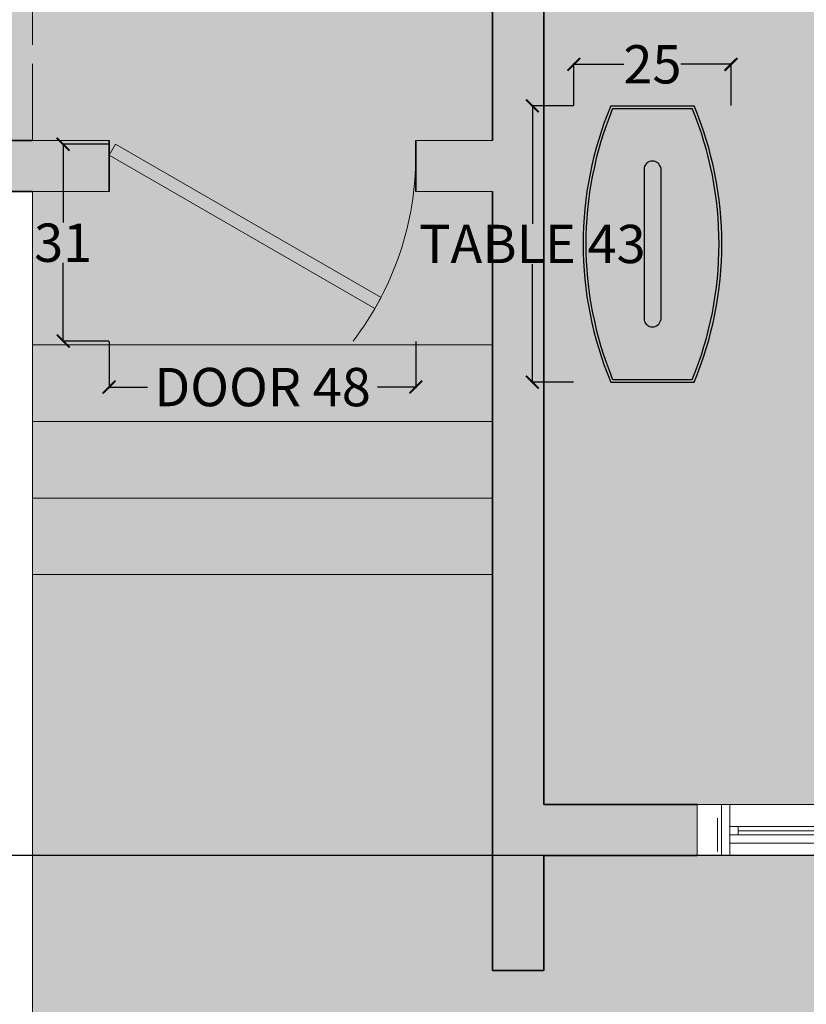
# Model space of a CAD drawing. Units: inches. Extents: x 1704 to 6393, y -157 to 1172.
# Tile 24 of 122: x 2275 to 2398, y 67 to 221. Entities that reach past the tile are written whole.
import ezdxf

# ---------------------------------------------------------------- set-up
doc = ezdxf.new("R2010")
doc.units = ezdxf.units.IN
doc.header["$MEASUREMENT"] = 0
doc.linetypes.add('ACAD_ISO02W100', pattern=[15, 12, -3])
for name, color, linetype, lineweight in [('A-ANNO-DIMS', 7, 'Continuous', 13), ('A-FURN', 8, 'Continuous', 18), ('A-WALL-OVHD', 8, 'ACAD_ISO02W100', 13), ('A-WALL-PATT', 7, 'Continuous', 13), ('DOORS', 160, 'Continuous', 18), ('L-HRDS', 8, 'Continuous', 18), ('STAIRS', 7, 'Continuous', 18), ('WALLS', 7, 'Continuous', 35), ('WINDOWS', 2, 'Continuous', 18)]:
    doc.layers.add(name, color=color, linetype=linetype, lineweight=lineweight)
doc.layers.add('A-FLOR-PATT', color=7, linetype='Continuous', lineweight=13, true_color=0xf2f2f2)
doc.layers.add('L-HRDS-PATT', color=9, linetype='Continuous', lineweight=13, true_color=0xc5c1ba)
doc.layers.add('MESA', color=7, linetype='Continuous')
doc.styles.get("Standard").update_dxf_attribs({"font": 'arial.ttf'})
doc.dimstyles.get("Standard").update_dxf_attribs({"dimtxt": 6, "dimasz": 2, "dimexe": 0.18, "dimexo": 0.0625, "dimgap": 0.09, "dimtad": 0, "dimtih": 1, "dimtoh": 1, "dimdec": 1, "dimzin": 0, "dimdsep": 46, "dimlunit": 3, "dimtxsty": 'Standard', "dimblk": 'ARCHTICK', "dimcen": 0.09, "dimadec": 0, "dimazin": 0, "dimtfac": 1, "dimtdec": 1, "dimtofl": 0, "dimtmove": 0, "dimatfit": 3, "dimfxl": 1, "dimtolj": 1, "dimtzin": 0, "dimarcsym": 0})

# ---------------------------------------------------------------- blocks, each defined once
blk = doc.blocks.new('Door - Left Hung 36 in.')
blk.add_lwpolyline([(0.75, -1.3), (0, 0), (31.18, 18), (31.93, 16.7)], close=True)
blk.add_arc((0, 0), 36, 0, 37.3101)
blk = doc.blocks.new('Mesa Double Face')
at = {"layer": 'MESA', "ltscale": 0.8}
h = blk.add_hatch(color=256, dxfattribs=at)
h.dxf.hatch_style = 1
h.set_gradient(color1=(7, 8, 8), color2=(0, 0, 0), one_color=1, name='CYLINDER')
h.paths.add_polyline_path([(0.3, 0), (-0.3, 0, 0.200446), (-0.3, -1.9938), (0.3, -1.9938, 0.200446)])
h.paths.add_polyline_path([(0.2866, -0.02, -0.197751), (0.2866, -1.9738), (-0.2866, -1.9738, -0.197751), (-0.2866, -0.02)], flags=16)
h.paths.add_polyline_path([(-0.05, -1.6469, 0.951918), (0.05, -1.6469), (0.05, -0.3469, 0.951918), (-0.05, -0.3469)], flags=0)
h = blk.add_hatch(color=256, dxfattribs=at)
h.dxf.hatch_style = 1
h.set_gradient(color1=(131, 90, 73), color2=(169, 122, 102), one_color=1, tint=0.53, name='CYLINDER')
h.paths.add_polyline_path([(0.2866, -0.02), (-0.2866, -0.02, 0.197751), (-0.2866, -1.9738), (0.2866, -1.9738, 0.197751)])
h.paths.add_polyline_path([(-0.06, -1.5469, 0.793265), (0.06, -1.5469), (0.06, -0.4469, 0.793265), (-0.06, -0.4469)], flags=16)
h = blk.add_hatch(color=256, dxfattribs=at)
h.dxf.hatch_style = 1
h.set_gradient(color1=(7, 8, 8), color2=(0, 0, 0), one_color=1, name='CYLINDER')
h.paths.add_polyline_path([(0.06, -0.4469, 0.793265), (-0.06, -0.4469), (-0.06, -1.5469, 0.793265), (0.06, -1.5469)])
for p, q in [((-0.3, 0), (0.3, 0)), ((-0.2866, -0.02), (0.2866, -0.02)), ((-0.06, -0.4469), (-0.06, -1.5469)), ((0.06, -0.4469), (0.06, -1.5469)), ((-0.2866, -1.9738), (0.2866, -1.9738)), ((-0.3, -1.9938), (0.3, -1.9938))]:
    blk.add_line(p, q, dxfattribs=at)
for centre, radius, start, end in [((2.0867, -0.9969), 2.5866, 157.33098, 202.66902), ((2.0867, -0.9969), 2.5666, 157.62803, 202.37197), ((-2.0867, -0.9969), 2.5666, 337.62803, 22.37197), ((-2.0867, -0.9969), 2.5866, 337.33098, 22.66902), ((0, -0.4609), 0.0616, 13.15255, 166.84745), ((0, -1.5329), 0.0616, 193.15255, 346.84745)]:
    blk.add_arc(centre, radius, start, end, dxfattribs=at)
blk = doc.blocks.new('WIN-SLIDER-48')
for p, q in [((3.83, 8), (0, 8)), ((5.13, 8), (42.87, 8)), ((44.17, 8), (48, 8)), ((3.18, 5.86), (3.18, 0.65)), ((44.82, 5.86), (44.82, 0.65)), ((6.43, 4.55), (22.7, 4.55)), ((6.43, 3.9), (22.7, 3.9)), ((6.43, 3.25), (22.7, 3.25)), ((24, 4.55), (42.87, 4.55)), ((25.3, 3.9), (28.1, 3.9)), ((25.3, 3.25), (41.56, 3.25)), ((24, 1.95), (5.13, 1.95)), ((22.7, 2.6), (19.9, 2.6)), ((25.3, 2.6), (41.56, 2.6)), ((25.3, 1.95), (41.56, 1.95)), ((3.83, 0), (0, 0)), ((5.13, 0), (42.87, 0)), ((44.17, 0), (48, 0))]:
    blk.add_line(p, q)
for points in [[(5.13, 0), (3.83, 0), (3.83, 8), (5.13, 8)], [(42.87, 0), (44.17, 0), (44.17, 8), (42.87, 8)], [(5.13, 3.25), (6.43, 3.25), (6.43, 4.55), (5.13, 4.55)], [(22.7, 3.25), (24, 3.25), (24, 4.55), (22.7, 4.55)], [(24, 1.95), (25.3, 1.95), (25.3, 3.25), (24, 3.25)], [(28.43, 3.9), (28.1, 4.1), (28.1, 3.71)], [(41.56, 1.95), (42.87, 1.95), (42.87, 3.25), (41.56, 3.25)], [(19.57, 2.6), (19.9, 2.8), (19.9, 2.41)]]:
    blk.add_lwpolyline(points, close=True)
blk = doc.blocks.new('_ArchTick')
at = {"color": 0, "linetype": 'ByBlock', "const_width": 0.15}
blk.add_lwpolyline([(-0.5, -0.5), (0.5, 0.5)], dxfattribs=at)
blk = doc.blocks.new('*D28')
at = {"layer": 'A-ANNO-DIMS', "color": 0, "lineweight": -2, "transparency": 16777216}
for p, q in [((2289.35, 170.73), (2289.35, 163.41)), ((2337.35, 170.73), (2337.35, 163.41)), ((2289.35, 163.59), (2295.37, 163.59)), ((2337.35, 163.59), (2331.33, 163.59))]:
    blk.add_line(p, q, dxfattribs=at)
at = {"layer": 'Defpoints', "color": 0, "lineweight": -3, "transparency": 16777216}
for p in [(2289.35, 170.79), (2337.35, 170.79), (2337.35, 163.59)]:
    blk.add_point(p, dxfattribs=at)
at = {"layer": 'A-ANNO-DIMS', "color": 0, "lineweight": -2, "transparency": 16777216, "xscale": 2, "yscale": 2, "zscale": 2, "rotation": 180}
blk.add_blockref('_ArchTick', (2289.35, 163.59), dxfattribs=at)
at = {"layer": 'A-ANNO-DIMS', "color": 0, "lineweight": -2, "transparency": 16777216, "xscale": 2, "yscale": 2, "zscale": 2}
blk.add_blockref('_ArchTick', (2337.35, 163.59), dxfattribs=at)
at = {"layer": 'A-ANNO-DIMS', "color": 0, "transparency": 16777216, "insert": (2313.35, 163.59), "char_height": 6, "attachment_point": 5}
blk.add_mtext('\\A1;DOOR 48', dxfattribs=at)
blk = doc.blocks.new('*D29')
at = {"layer": 'A-ANNO-DIMS', "color": 0, "lineweight": -2, "transparency": 16777216}
for p, q in [((2289.29, 201.62), (2281.97, 201.62)), ((2282.15, 201.62), (2282.15, 189.36)), ((2282.15, 170.79), (2282.15, 183.05)), ((2289.29, 170.79), (2281.97, 170.79))]:
    blk.add_line(p, q, dxfattribs=at)
at = {"layer": 'Defpoints', "color": 0, "lineweight": -3, "transparency": 16777216}
for p in [(2289.35, 201.62), (2282.15, 170.79), (2289.35, 170.79)]:
    blk.add_point(p, dxfattribs=at)
at = {"layer": 'A-ANNO-DIMS', "color": 0, "lineweight": -2, "transparency": 16777216, "xscale": 2, "yscale": 2, "zscale": 2}
for p, rotation in [((2282.15, 201.62), 90), ((2282.15, 170.79), 270)]:
    blk.add_blockref('_ArchTick', p, dxfattribs=dict(at, rotation=rotation))
at = {"layer": 'A-ANNO-DIMS', "color": 0, "transparency": 16777216, "insert": (2282.15, 186.2), "char_height": 6, "attachment_point": 5}
blk.add_mtext('\\A1;31', dxfattribs=at)
blk = doc.blocks.new('*D66')
at = {"layer": 'A-ANNO-DIMS', "color": 0, "lineweight": -2, "transparency": 16777216}
for p, q in [((2362.01, 207.65), (2355.4, 207.65)), ((2355.58, 207.65), (2355.58, 189.16)), ((2355.58, 164.36), (2355.58, 182.85)), ((2362.01, 164.36), (2355.4, 164.36))]:
    blk.add_line(p, q, dxfattribs=at)
at = {"layer": 'Defpoints', "color": 0, "lineweight": -3, "transparency": 16777216}
for p in [(2355.58, 207.65), (2362.07, 207.65), (2362.07, 164.36)]:
    blk.add_point(p, dxfattribs=at)
at = {"layer": 'A-ANNO-DIMS', "color": 0, "lineweight": -2, "transparency": 16777216, "xscale": 2, "yscale": 2, "zscale": 2}
for p, rotation in [((2355.58, 207.65), 90), ((2355.58, 164.36), 270)]:
    blk.add_blockref('_ArchTick', p, dxfattribs=dict(at, rotation=rotation))
at = {"layer": 'A-ANNO-DIMS', "color": 0, "transparency": 16777216, "insert": (2355.58, 186), "char_height": 6, "attachment_point": 5}
blk.add_mtext('\\A1;TABLE 43', dxfattribs=at)
blk = doc.blocks.new('*D67')
at = {"layer": 'A-ANNO-DIMS', "color": 0, "lineweight": -2, "transparency": 16777216}
for p, q in [((2362.07, 207.71), (2362.07, 214.32)), ((2362.07, 214.14), (2369.91, 214.14)), ((2386.67, 214.14), (2378.83, 214.14)), ((2386.67, 207.71), (2386.67, 214.32))]:
    blk.add_line(p, q, dxfattribs=at)
at = {"layer": 'Defpoints', "color": 0, "lineweight": -3, "transparency": 16777216}
for p in [(2386.67, 214.14), (2362.07, 207.65), (2386.67, 207.65)]:
    blk.add_point(p, dxfattribs=at)
at = {"layer": 'A-ANNO-DIMS', "color": 0, "lineweight": -2, "transparency": 16777216, "xscale": 2, "yscale": 2, "zscale": 2, "rotation": 180}
blk.add_blockref('_ArchTick', (2362.07, 214.14), dxfattribs=at)
at = {"layer": 'A-ANNO-DIMS', "color": 0, "lineweight": -2, "transparency": 16777216, "xscale": 2, "yscale": 2, "zscale": 2}
blk.add_blockref('_ArchTick', (2386.67, 214.14), dxfattribs=at)
at = {"layer": 'A-ANNO-DIMS', "color": 0, "transparency": 16777216, "insert": (2374.37, 214.14), "char_height": 6, "attachment_point": 5}
blk.add_mtext('\\A1;25', dxfattribs=at)
blk = doc.blocks.new('*D93')
at = {"layer": 'A-ANNO-DIMS', "color": 0, "lineweight": -2, "transparency": 16777216}
for p, q in [((2605.29, 895.21), (1829.7, 895.21)), ((1829.88, 895.21), (1829.88, 495.87)), ((1829.88, 90.21), (1829.88, 489.56)), ((2605.29, 90.21), (1829.7, 90.21))]:
    blk.add_line(p, q, dxfattribs=at)
at = {"layer": 'Defpoints', "color": 0, "lineweight": -3, "transparency": 16777216}
for p in [(2605.35, 895.21), (1829.88, 90.21), (2605.35, 90.21)]:
    blk.add_point(p, dxfattribs=at)
at = {"layer": 'A-ANNO-DIMS', "color": 0, "lineweight": -2, "transparency": 16777216, "xscale": 2, "yscale": 2, "zscale": 2}
for p, rotation in [((1829.88, 895.21), 90), ((1829.88, 90.21), 270)]:
    blk.add_blockref('_ArchTick', p, dxfattribs=dict(at, rotation=rotation))
at = {"layer": 'A-ANNO-DIMS', "color": 0, "transparency": 16777216, "insert": (1829.88, 492.71), "char_height": 6, "attachment_point": 5}
blk.add_mtext('\\A1;805', dxfattribs=at)

msp = doc.modelspace()

# ---------------------------------------------------------------- hatches: boundary and pattern name
at = {"layer": 'A-FLOR-PATT', "transparency": 33554528}
h = msp.add_hatch(color=256, dxfattribs=at)
h.dxf.hatch_style = 1
h.paths.add_polyline_path([(2325.349, 863.213), (2325.349, 887.213), (2263.349, 887.213), (2167.349, 887.213), (2081.349, 887.213), (2081.349, 719.213), (2277.349, 719.213), (2277.349, 711.213), (2277.349, 372.213), (2349.349, 372.213), (2381.349, 372.213), (2381.349, 364.213), (2353.349, 364.213), (2353.349, 270.213), (2381.349, 270.213), (2381.349, 266.213), (2357.349, 266.213), (2357.349, 98.213), (2381.349, 98.213), (2385.181, 98.213), (2386.482, 98.213), (2424.215, 98.213), (2425.516, 98.213), (2429.349, 98.213), (2597.349, 98.213), (2597.349, 146.213), (2597.349, 218.213), (2597.349, 266.213), (2423.349, 266.213), (2423.349, 270.213), (2473.349, 270.213), (2473.349, 294.213), (2477.349, 294.213), (2477.349, 270.213), (2547.349, 270.213), (2547.349, 364.213), (2477.349, 364.213), (2477.349, 318.213), (2473.349, 318.213), (2473.349, 364.213), (2423.349, 364.213), (2423.349, 372.213), (2469.349, 372.213), (2469.349, 459.213), (2469.349, 538.213), (2350.349, 538.213), (2350.349, 565.713), (2358.349, 565.713), (2358.349, 545.213), (2420.349, 545.213), (2420.349, 610.213), (2358.349, 610.213), (2358.349, 589.713), (2350.349, 589.713), (2350.349, 615.213), (2425.349, 615.213), (2425.349, 607.213), (2425.349, 546.213), (2469.349, 546.213), (2514.349, 546.213), (2514.349, 607.213), (2449.349, 607.213), (2449.349, 615.213), (2451.738, 615.213), (2451.738, 659.213), (2427.738, 659.213), (2427.738, 665.213), (2367.738, 665.213), (2367.738, 667.213), (2367.738, 711.213), (2325.349, 711.213), (2325.349, 719.213), (2325.349, 755.213), (2325.349, 763.213)])
h.paths.add_polyline_path([(2233.858, 822.533, -0.187247), (2233.858, 809.14), (2231.697, 808.804, 0.0848928), (2233.131, 814.486), (2230.424, 814.486, -0.1042581), (2228.553, 808.313), (2217.751, 807.156, -0.2222222), (2217.751, 824.517), (2228.553, 823.359, -0.1042581), (2230.424, 817.186), (2233.131, 817.186, 0.0848928), (2231.697, 822.868)], flags=16)
h.paths.add_polyline_path([(2213.621, 833.197), (2213.621, 798.475), (2156.048, 798.475), (2156.048, 833.197)], flags=16)
h.paths.add_polyline_path([(2203.932, 848.099), (2205.089, 837.296, -0.2222222), (2187.728, 837.296), (2188.885, 848.099, -0.1042581), (2195.058, 849.969), (2195.058, 852.676, 0.0848928), (2189.377, 851.242), (2189.712, 853.404, -0.187247), (2203.105, 853.404), (2203.44, 851.242, 0.0848928), (2197.759, 852.676), (2197.759, 849.969, -0.1042581)], flags=16)
h.paths.add_polyline_path([(2181.941, 837.296, -0.2222222), (2164.58, 837.296), (2165.737, 848.099, -0.1042581), (2171.91, 849.969), (2171.91, 852.676, 0.0848928), (2166.229, 851.242), (2166.564, 853.404, -0.187247), (2179.957, 853.404), (2180.292, 851.242, 0.0848928), (2174.611, 852.676), (2174.611, 849.969, -0.1042581), (2180.784, 848.099)], flags=16)
h.paths.add_polyline_path([(2205.089, 794.376), (2203.932, 783.574, -0.1042581), (2197.759, 781.703), (2197.759, 778.996, 0.0848928), (2203.44, 780.43), (2203.105, 778.269, -0.187247), (2189.712, 778.269), (2189.377, 780.43, 0.0848928), (2195.058, 778.996), (2195.058, 781.703, -0.1042581), (2188.885, 783.574), (2187.728, 794.376, -0.2222222)], flags=16)
h.paths.add_polyline_path([(2181.941, 794.376), (2180.784, 783.574, -0.1042581), (2174.611, 781.703), (2174.611, 778.996, 0.0848928), (2180.292, 780.43), (2179.957, 778.269, -0.187247), (2166.564, 778.269), (2166.229, 780.43, 0.0848928), (2171.91, 778.996), (2171.91, 781.703, -0.1042581), (2165.737, 783.574), (2164.58, 794.376, -0.2222222)], flags=16)
h.paths.add_polyline_path([(2151.918, 807.156), (2141.116, 808.313, -0.1042581), (2139.245, 814.486), (2136.539, 814.486, 0.0848928), (2137.972, 808.804), (2135.811, 809.14, -0.187247), (2135.811, 822.533), (2137.972, 822.868, 0.0848928), (2136.539, 817.186), (2139.245, 817.186, -0.1042581), (2141.116, 823.359), (2151.918, 824.517, -0.2222222)], flags=16)
h.paths.add_polyline_path([(2357.868, 363.41), (2358.814, 363.41, 0.7537605)], flags=16)
h.paths.add_polyline_path([(2372.241, 363.117), (2372.248, 363.117), (2372.248, 363.343), (2371.302, 363.343), (2371.302, 363.139, -1.3603913)], flags=16)
h.paths.add_polyline_path([(2371.309, 272.716), (2371.302, 272.716), (2371.302, 272.49), (2372.248, 272.49), (2372.248, 272.693, -1.3603913)], flags=16)
h.paths.add_polyline_path([(2357.875, 272.716), (2357.868, 272.716), (2357.868, 272.49), (2358.814, 272.49), (2358.814, 272.693, -1.3603913)], flags=16)
h.paths.add_polyline_path([(2353.769, 363.074), (2376.347, 363.074), (2376.347, 272.759), (2353.769, 272.759)], flags=16)
h.paths.add_polyline_path([(2354.772, 362.07), (2375.344, 362.07), (2375.344, 273.762), (2354.772, 273.762)], flags=0)
h.paths.add_polyline_path([(2357.868, 363.343), (2358.814, 363.343), (2358.814, 363.117), (2357.868, 363.117)], flags=16)
h.paths.add_polyline_path([(2359.288, 359.184), (2359.288, 360.063), (2370.828, 360.063), (2370.828, 359.184), (2374.332, 359.184), (2374.332, 358.464), (2372.835, 358.464), (2372.835, 357.541), (2374.332, 357.541), (2374.332, 356.82), (2372.835, 356.82), (2372.835, 355.898), (2374.332, 355.898), (2374.332, 355.177), (2372.835, 355.177), (2372.835, 354.254), (2374.332, 354.254), (2374.332, 353.534), (2372.835, 353.534), (2372.835, 352.611), (2374.332, 352.611), (2374.332, 351.89), (2372.835, 351.89), (2372.835, 350.968), (2374.332, 350.968), (2374.332, 350.247), (2372.835, 350.247), (2372.835, 349.324), (2374.332, 349.324), (2374.332, 348.604), (2372.835, 348.604), (2372.835, 347.681), (2374.332, 347.681), (2374.332, 346.96), (2372.835, 346.96), (2372.835, 346.038), (2374.332, 346.038), (2374.332, 345.317), (2372.835, 345.317), (2372.835, 344.395), (2374.332, 344.395), (2374.332, 343.674), (2372.835, 343.674), (2372.835, 342.751), (2374.332, 342.751), (2374.332, 342.03), (2372.835, 342.03), (2372.835, 341.108), (2374.332, 341.108), (2374.332, 340.387), (2372.835, 340.387), (2372.835, 339.465), (2374.332, 339.465), (2374.332, 338.744), (2372.835, 338.744), (2372.835, 337.821), (2374.332, 337.821), (2374.332, 337.1), (2372.835, 337.1), (2372.835, 336.178), (2374.332, 336.178), (2374.332, 335.457), (2372.835, 335.457), (2372.835, 334.535), (2374.332, 334.535), (2374.332, 333.814), (2372.835, 333.814), (2372.835, 332.891), (2374.332, 332.891), (2374.332, 332.171), (2372.835, 332.171), (2372.835, 331.248), (2374.332, 331.248), (2374.332, 330.527), (2372.835, 330.527), (2372.835, 329.605), (2374.332, 329.605), (2374.332, 328.884), (2372.835, 328.884), (2372.835, 327.961), (2374.332, 327.961), (2374.332, 327.241), (2372.835, 327.241), (2372.835, 326.318), (2374.332, 326.318), (2374.332, 325.597), (2372.835, 325.597), (2372.835, 324.675), (2374.332, 324.675), (2374.332, 323.954), (2372.835, 323.954), (2372.835, 323.031), (2374.332, 323.031), (2374.332, 322.311), (2372.835, 322.311), (2372.835, 321.388), (2374.332, 321.388), (2374.332, 320.667), (2372.835, 320.667), (2372.835, 319.745), (2374.332, 319.745), (2374.332, 319.024), (2372.835, 319.024), (2372.835, 318.102), (2374.332, 318.102), (2374.332, 317.381), (2372.835, 317.381), (2372.835, 316.458), (2374.332, 316.458), (2374.332, 315.737), (2372.835, 315.737), (2372.835, 314.815), (2374.332, 314.815), (2374.332, 314.094), (2372.835, 314.094), (2372.835, 313.172), (2374.332, 313.172), (2374.332, 312.451), (2372.835, 312.451), (2372.835, 311.528), (2374.332, 311.528), (2374.332, 310.807), (2372.835, 310.807), (2372.835, 309.885), (2374.332, 309.885), (2374.332, 309.164), (2372.835, 309.164), (2372.835, 308.242), (2374.332, 308.242), (2374.332, 307.521), (2372.835, 307.521), (2372.835, 306.598), (2374.332, 306.598), (2374.332, 305.878), (2372.835, 305.878), (2372.835, 304.955), (2374.332, 304.955), (2374.332, 304.234), (2372.835, 304.234), (2372.835, 303.312), (2374.332, 303.312), (2374.332, 302.591), (2372.835, 302.591), (2372.835, 301.668), (2374.332, 301.668), (2374.332, 300.948), (2372.835, 300.948), (2372.835, 300.025), (2374.332, 300.025), (2374.332, 299.304), (2372.835, 299.304), (2372.835, 298.382), (2374.332, 298.382), (2374.332, 297.661), (2372.835, 297.661), (2372.835, 296.738), (2374.332, 296.738), (2374.332, 296.018), (2372.835, 296.018), (2372.835, 295.095), (2374.332, 295.095), (2374.332, 294.374), (2372.835, 294.374), (2372.835, 293.452), (2374.332, 293.452), (2374.332, 292.731), (2372.835, 292.731), (2372.835, 291.809), (2374.332, 291.809), (2374.332, 291.088), (2372.835, 291.088), (2372.835, 290.165), (2374.332, 290.165), (2374.332, 289.444), (2372.835, 289.444), (2372.835, 288.522), (2374.332, 288.522), (2374.332, 287.801), (2372.835, 287.801), (2372.835, 286.879), (2374.332, 286.879), (2374.332, 286.158), (2372.835, 286.158), (2372.835, 285.235), (2374.332, 285.235), (2374.332, 284.514), (2372.835, 284.514), (2372.835, 283.592), (2374.332, 283.592), (2374.332, 282.871), (2372.835, 282.871), (2372.835, 281.949), (2374.332, 281.949), (2374.332, 281.228), (2372.835, 281.228), (2372.835, 280.305), (2374.332, 280.305), (2374.332, 279.585), (2372.835, 279.585), (2372.835, 278.662), (2374.332, 278.662), (2374.332, 277.941), (2372.835, 277.941), (2372.835, 277.019), (2374.332, 277.019), (2374.332, 276.298), (2370.828, 276.298), (2370.828, 275.769), (2359.288, 275.769), (2359.288, 276.298), (2355.784, 276.298), (2355.784, 277.019), (2357.281, 277.019), (2357.281, 277.941), (2355.784, 277.941), (2355.784, 278.662), (2357.281, 278.662), (2357.281, 279.585), (2355.784, 279.585), (2355.784, 280.305), (2357.281, 280.305), (2357.281, 281.228), (2355.784, 281.228), (2355.784, 281.949), (2357.281, 281.949), (2357.281, 282.871), (2355.784, 282.871), (2355.784, 283.592), (2357.281, 283.592), (2357.281, 284.514), (2355.784, 284.514), (2355.784, 285.235), (2357.281, 285.235), (2357.281, 286.158), (2355.784, 286.158), (2355.784, 286.879), (2357.281, 286.879), (2357.281, 287.801), (2355.784, 287.801), (2355.784, 288.522), (2357.281, 288.522), (2357.281, 289.444), (2355.784, 289.444), (2355.784, 290.165), (2357.281, 290.165), (2357.281, 291.088), (2355.784, 291.088), (2355.784, 291.809), (2357.281, 291.809), (2357.281, 292.731), (2355.784, 292.731), (2355.784, 293.452), (2357.281, 293.452), (2357.281, 294.374), (2355.784, 294.374), (2355.784, 295.095), (2357.281, 295.095), (2357.281, 296.018), (2355.784, 296.018), (2355.784, 296.738), (2357.281, 296.738), (2357.281, 297.661), (2355.784, 297.661), (2355.784, 298.382), (2357.281, 298.382), (2357.281, 299.304), (2355.784, 299.304), (2355.784, 300.025), (2357.281, 300.025), (2357.281, 300.948), (2355.784, 300.948), (2355.784, 301.668), (2357.281, 301.668), (2357.281, 302.591), (2355.784, 302.591), (2355.784, 303.312), (2357.281, 303.312), (2357.281, 304.234), (2355.784, 304.234), (2355.784, 304.955), (2357.281, 304.955), (2357.281, 305.878), (2355.784, 305.878), (2355.784, 306.598), (2357.281, 306.598), (2357.281, 307.521), (2355.784, 307.521), (2355.784, 308.242), (2357.281, 308.242), (2357.281, 309.164), (2355.784, 309.164), (2355.784, 309.885), (2357.281, 309.885), (2357.281, 310.807), (2355.784, 310.807), (2355.784, 311.528), (2357.281, 311.528), (2357.281, 312.451), (2355.784, 312.451), (2355.784, 313.172), (2357.281, 313.172), (2357.281, 314.094), (2355.784, 314.094), (2355.784, 314.815), (2357.281, 314.815), (2357.281, 315.737), (2355.784, 315.737), (2355.784, 316.458), (2357.281, 316.458), (2357.281, 317.381), (2355.784, 317.381), (2355.784, 318.102), (2357.281, 318.102), (2357.281, 319.024), (2355.784, 319.024), (2355.784, 319.745), (2357.281, 319.745), (2357.281, 320.667), (2355.784, 320.667), (2355.784, 321.388), (2357.281, 321.388), (2357.281, 322.311), (2355.784, 322.311), (2355.784, 323.031), (2357.281, 323.031), (2357.281, 323.954), (2355.784, 323.954), (2355.784, 324.675), (2357.281, 324.675), (2357.281, 325.597), (2355.784, 325.597), (2355.784, 326.318), (2357.281, 326.318), (2357.281, 327.241), (2355.784, 327.241), (2355.784, 327.961), (2357.281, 327.961), (2357.281, 328.884), (2355.784, 328.884), (2355.784, 329.605), (2357.281, 329.605), (2357.281, 330.527), (2355.784, 330.527), (2355.784, 331.248), (2357.281, 331.248), (2357.281, 332.171), (2355.784, 332.171), (2355.784, 332.891), (2357.281, 332.891), (2357.281, 333.814), (2355.784, 333.814), (2355.784, 334.535), (2357.281, 334.535), (2357.281, 335.457), (2355.784, 335.457), (2355.784, 336.178), (2357.281, 336.178), (2357.281, 337.1), (2355.784, 337.1), (2355.784, 337.821), (2357.281, 337.821), (2357.281, 338.744), (2355.784, 338.744), (2355.784, 339.465), (2357.281, 339.465), (2357.281, 340.387), (2355.784, 340.387), (2355.784, 341.108), (2357.281, 341.108), (2357.281, 342.03), (2355.784, 342.03), (2355.784, 342.751), (2357.281, 342.751), (2357.281, 343.674), (2355.784, 343.674), (2355.784, 344.395), (2357.281, 344.395), (2357.281, 345.317), (2355.784, 345.317), (2355.784, 346.038), (2357.281, 346.038), (2357.281, 346.96), (2355.784, 346.96), (2355.784, 347.681), (2357.281, 347.681), (2357.281, 348.604), (2355.784, 348.604), (2355.784, 349.324), (2357.281, 349.324), (2357.281, 350.247), (2355.784, 350.247), (2355.784, 350.968), (2357.281, 350.968), (2357.281, 351.89), (2355.784, 351.89), (2355.784, 352.611), (2357.281, 352.611), (2357.281, 353.534), (2355.784, 353.534), (2355.784, 354.254), (2357.281, 354.254), (2357.281, 355.177), (2355.784, 355.177), (2355.784, 355.898), (2357.281, 355.898), (2357.281, 356.82), (2355.784, 356.82), (2355.784, 357.541), (2357.281, 357.541), (2357.281, 358.464), (2355.784, 358.464), (2355.784, 359.184)], flags=0)
h = msp.add_hatch(color=256, dxfattribs=at)
h.dxf.hatch_style = 1
h.paths.add_polyline_path([(2349.349, 372.213), (2277.349, 372.213), (2277.349, 364.213), (2349.349, 364.213)])
h.paths.add_polyline_path([(2277.349, 372.213), (2273.349, 372.213), (2273.349, 364.213), (2277.349, 364.213)])
h.paths.add_polyline_path([(2277.349, 364.213), (2273.349, 364.213), (2273.349, 202.213), (2277.349, 202.213)])
h.paths.add_polyline_path([(2277.349, 538.213), (2273.349, 538.213), (2273.349, 372.213), (2277.349, 372.213)])
h.paths.add_polyline_path([(2277.349, 629.213), (2273.349, 629.213), (2273.349, 545.213), (2277.349, 545.213)])
h.paths.add_polyline_path([(2277.349, 711.213), (2273.349, 711.213), (2273.349, 631.213), (2277.349, 631.213)])
h.paths.add_polyline_path([(2277.349, 631.213), (2273.349, 631.213), (2273.349, 629.213), (2277.349, 629.213)])
at = {"layer": 'A-WALL-PATT', "transparency": 33554643}
h = msp.add_hatch(color=256, dxfattribs=at)
h.dxf.hatch_style = 1
h.paths.add_polyline_path([(2167.349, 895.213), (2073.349, 895.213), (2073.349, 887.213), (2081.349, 887.213), (2167.349, 887.213)])
h.paths.add_polyline_path([(2465.349, 895.213), (2273.349, 895.213), (2273.349, 903.213), (2263.349, 903.213), (2263.349, 895.213), (2263.349, 887.213), (2325.349, 887.213), (2325.349, 863.213), (2333.349, 863.213), (2333.349, 887.213), (2465.349, 887.213)])
h.paths.add_polyline_path([(2533.349, 895.213), (2513.349, 895.213), (2513.349, 887.213), (2513.349, 861.213), (2517.349, 861.213), (2517.349, 887.213), (2533.349, 887.213)])
h.paths.add_polyline_path([(2605.349, 895.213), (2581.349, 895.213), (2581.349, 887.213), (2597.349, 887.213), (2597.349, 854.213), (2605.349, 854.213)])
h.paths.add_polyline_path([(2605.349, 752.213), (2629.349, 752.213), (2629.349, 716.213), (2605.349, 716.213), (2605.349, 712.213), (2719.349, 712.213), (2719.349, 716.213), (2631.349, 716.213), (2631.349, 754.213), (2605.349, 754.213), (2605.349, 794.213), (2597.349, 794.213), (2597.349, 787.213), (2517.349, 787.213), (2517.349, 813.213), (2513.349, 813.213), (2513.349, 783.213), (2517.349, 783.213), (2597.349, 783.213), (2597.349, 719.213), (2517.349, 719.213), (2517.349, 753.213), (2513.349, 753.213), (2513.349, 719.213), (2365.349, 719.213), (2365.349, 763.213), (2325.349, 763.213), (2325.349, 755.213), (2357.349, 755.213), (2357.349, 719.213), (2325.349, 719.213), (2325.349, 711.213), (2547.349, 711.213), (2547.349, 615.213), (2449.349, 615.213), (2449.349, 607.213), (2514.349, 607.213), (2514.349, 546.213), (2439.349, 546.213), (2425.349, 546.213), (2425.349, 607.213), (2425.349, 615.213), (2350.349, 615.213), (2350.349, 589.713), (2358.349, 589.713), (2358.349, 610.213), (2420.349, 610.213), (2420.349, 545.213), (2358.349, 545.213), (2358.349, 565.713), (2350.349, 565.713), (2350.349, 538.213), (2469.349, 538.213), (2469.349, 459.213), (2469.349, 372.213), (2423.349, 372.213), (2423.349, 364.213), (2473.349, 364.213), (2473.349, 318.213), (2477.349, 318.213), (2477.349, 364.213), (2547.349, 364.213), (2547.349, 352.213), (2549.349, 352.213), (2549.349, 364.213), (2597.349, 364.213), (2597.349, 328.213), (2549.349, 328.213), (2547.349, 328.213), (2547.349, 326.213), (2549.349, 326.213), (2597.349, 326.213), (2605.349, 326.213), (2605.349, 377.057), (2597.349, 377.057), (2597.349, 372.213), (2477.349, 372.213), (2477.349, 451.213), (2597.349, 451.213), (2605.349, 451.213), (2605.349, 459.213), (2597.349, 459.213), (2477.349, 459.213), (2477.349, 538.213), (2597.349, 538.213), (2597.349, 495.213), (2605.349, 495.213), (2605.349, 512.213), (2631.349, 512.213), (2631.349, 568.213), (2605.349, 568.213), (2605.349, 577.213), (2597.349, 577.213), (2597.349, 542.213), (2518.349, 542.213), (2518.349, 607.213), (2532.349, 607.213), (2605.349, 607.213), (2605.349, 615.213), (2597.349, 615.213), (2551.349, 615.213), (2551.349, 711.213), (2597.349, 711.213), (2597.349, 645.213), (2605.349, 645.213), (2605.349, 712.213), (2605.349, 716.213)])
h.paths.add_polyline_path([(2605.349, 566.213), (2629.349, 566.213), (2629.349, 514.213), (2605.349, 514.213)], flags=16)
h.paths.add_polyline_path([(2381.349, 372.213), (2349.349, 372.213), (2349.349, 202.213), (2337.349, 202.213), (2337.349, 194.213), (2349.349, 194.213), (2349.349, 90.213), (2349.349, 72.213), (2357.349, 72.213), (2357.349, 90.213), (2381.349, 90.213), (2381.349, 98.213), (2357.349, 98.213), (2357.349, 266.213), (2381.349, 266.213), (2381.349, 270.213), (2353.349, 270.213), (2353.349, 364.213), (2381.349, 364.213)])
h.paths.add_polyline_path([(2605.349, 302.213), (2597.349, 302.213), (2597.349, 270.213), (2477.349, 270.213), (2477.349, 294.213), (2473.349, 294.213), (2473.349, 270.213), (2423.349, 270.213), (2423.349, 266.213), (2597.349, 266.213), (2597.349, 218.213), (2605.349, 218.213)])
h.paths.add_polyline_path([(2605.349, 146.213), (2597.349, 146.213), (2597.349, 98.213), (2429.349, 98.213), (2429.349, 90.213), (2597.349, 90.213), (2597.349, 72.213), (2605.349, 72.213), (2605.349, 90.213)])
h.paths.add_polyline_path([(2225.349, 202.213), (2049.349, 202.213), (2049.349, 194.213), (2225.349, 194.213)])
h.paths.add_polyline_path([(2289.349, 202.213), (2277.349, 202.213), (2273.349, 202.213), (2269.516, 202.213), (2269.516, 194.213), (2273.349, 194.213), (2277.349, 194.213), (2289.349, 194.213)])
h.paths.add_polyline_path([(2273.349, 372.213), (2029.19, 372.213), (2029.19, 364.213), (2273.349, 364.213)])
h.paths.add_polyline_path([(2277.349, 545.213), (2213.349, 545.213), (2213.349, 573.213), (2205.349, 573.213), (2177.349, 573.213), (2177.349, 545.213), (2073.349, 545.213), (2073.349, 538.213), (2081.349, 538.213), (2277.349, 538.213)])
h.paths.add_polyline_path([(2181.349, 545.213), (2181.349, 569.213), (2205.349, 569.213), (2205.349, 545.213)], flags=16)
h.paths.add_polyline_path([(2277.349, 719.213), (2081.349, 719.213), (2073.349, 719.213), (2073.349, 711.213), (2154.575, 711.213), (2205.349, 711.213), (2205.349, 687.213), (2205.349, 629.213), (2213.349, 629.213), (2273.349, 629.213), (2273.349, 631.213), (2207.349, 631.213), (2207.349, 707.213), (2231.349, 707.213), (2231.349, 709.213), (2207.349, 709.213), (2207.349, 711.213), (2277.349, 711.213)])
at = {"layer": 'L-HRDS-PATT', "transparency": 33554539}
h = msp.add_hatch(color=256, dxfattribs=at)
h.dxf.hatch_style = 1
h.paths.add_polyline_path([(2651.217, 368.213), (2605.349, 368.213), (2605.349, 218.213), (2605.349, 212.464), (2605.349, 210.513), (2605.349, 153.913), (2605.349, 151.962), (2605.349, 146.213), (2605.349, 90.213), (2605.349, 72.213), (2601.349, 72.213), (2600.88, 50.634), (2719.349, 50.634), (2719.349, 72.213), (2711.349, 72.213), (2663.217, 72.213), (2651.217, 72.213)])
h.paths.add_polyline_path([(2711.349, 48.634), (2600.88, 48.634), (2576.88, 48.634), (2576.88, 17.658), (2711.349, 17.658)])
h.paths.add_polyline_path([(2601.349, 72.213), (2597.349, 72.213), (2597.349, 90.213), (2429.349, 90.213), (2425.516, 90.213), (2424.215, 90.213), (2386.482, 90.213), (2385.181, 90.213), (2381.349, 90.213), (2357.349, 90.213), (2357.349, 72.213), (2349.349, 72.213), (2349.349, 90.213), (2349.349, 134.213), (2277.349, 134.213), (2277.349, 50.634), (2566.88, 50.634), (2600.88, 50.634)])
h.paths.add_polyline_path([(2349.349, 146.213), (2277.349, 146.213), (2277.349, 134.213), (2349.349, 134.213)])
h.paths.add_polyline_path([(2349.349, 158.213), (2277.349, 158.213), (2277.349, 146.213), (2349.349, 146.213)])
h.paths.add_polyline_path([(2349.349, 170.213), (2277.349, 170.213), (2277.349, 158.213), (2349.349, 158.213)])
h.paths.add_polyline_path([(2349.349, 194.213), (2337.349, 194.213), (2337.349, 202.213), (2349.349, 202.213), (2349.349, 364.213), (2277.349, 364.213), (2277.349, 202.213), (2289.349, 202.213), (2289.349, 194.213), (2277.349, 194.213), (2277.349, 170.213), (2349.349, 170.213)])

# ---------------------------------------------------------------- linework, layer by layer
at = {"layer": 'A-WALL-OVHD'}
for p, q in [((2277.349, 202.213), (2277.349, 711.213)), ((2277.349, 202.213), (2289.349, 202.213)), ((2337.349, 202.213), (2349.349, 202.213)), ((2277.349, 194.213), (2289.349, 194.213)), ((2337.349, 194.213), (2349.349, 194.213))]:
    msp.add_line(p, q, dxfattribs=at)
at = {"layer": 'L-HRDS'}
msp.add_line((2277.349, 194.213), (2277.349, -3.787), dxfattribs=at)
at = {"layer": 'STAIRS'}
for p, q in [((2277.349, 170.213), (2349.349, 170.213)), ((2277.349, 158.213), (2349.349, 158.213)), ((2277.349, 158.213), (2349.349, 158.213)), ((2277.349, 146.213), (2349.349, 146.213)), ((2277.349, 146.213), (2349.349, 146.213)), ((2277.349, 134.213), (2349.349, 134.213)), ((2277.349, 134.213), (2349.349, 134.213))]:
    msp.add_line(p, q, dxfattribs=at)
at = {"layer": 'WALLS'}
for p, q in [((2349.349, 202.213), (2349.349, 372.213)), ((2357.349, 98.213), (2357.349, 266.213)), ((2277.349, 202.213), (2273.349, 202.213)), ((2289.349, 202.213), (2289.349, 194.213)), ((2337.349, 202.213), (2337.349, 194.213)), ((2277.349, 194.213), (2273.349, 194.213)), ((2349.349, 90.213), (2349.349, 194.213)), ((2381.349, 98.213), (2357.349, 98.213)), ((2349.349, 90.213), (2349.349, 72.213)), ((2357.349, 90.213), (2357.349, 72.213)), ((2381.349, 90.213), (2357.349, 90.213)), ((2349.349, 72.213), (2357.349, 72.213))]:
    msp.add_line(p, q, dxfattribs=at)
at = {"layer": 'WINDOWS'}
msp.add_line((2381.349, 98.213), (2381.349, 90.213), dxfattribs=at)

# ---------------------------------------------------------------- block references
at = {"layer": 'A-FURN', "xscale": 21.71466577978878, "yscale": 21.71466577978878, "zscale": 21.71466577978878}
msp.add_blockref('Mesa Double Face', (2374.37, 207.65), dxfattribs=at)
at = {"layer": 'DOORS', "xscale": -1.333333333333328, "yscale": 1.333333333333328, "zscale": 1.333333333333328, "rotation": 180}
msp.add_blockref('Door - Left Hung 36 in.', (2289.349, 199.886), dxfattribs=at)
at = {"layer": 'WINDOWS'}
msp.add_blockref('WIN-SLIDER-48', (2381.349, 90.213), dxfattribs=at)

# ---------------------------------------------------------------- dimensions: what is measured, and where the dimension line sits
at = {"layer": 'A-ANNO-DIMS'}
for base, p1, p2, angle, picture, middle in [((1829.878, 90.213), (2605.349, 895.213), (2605.349, 90.213), 90, '*D93', (1829.878, 492.713)), ((2282.149, 170.792), (2289.349, 201.618), (2289.349, 170.792), 270, '*D29', (2282.149, 186.205))]:
    dim = msp.add_linear_dim(base=base, p1=p1, p2=p2, angle=angle, dimstyle='Standard', override={"dimdec": 0, "dimlfac": 1, "dimrnd": 0, "dimzin": 0, "dimdsep": 46, "dimlunit": 2}, dxfattribs=at)
    dim.commit()
    dim.dimension.update_dxf_attribs({"geometry": picture, "text_midpoint": middle})
dim = msp.add_linear_dim(base=(2386.67, 214.144), p1=(2362.07, 207.65), p2=(2386.67, 207.65), dimstyle='Standard', override={"dimdec": 0, "dimlfac": 1, "dimrnd": 0, "dimzin": 0, "dimdsep": 46, "dimlunit": 2}, dxfattribs=at)
dim.commit()
dim.dimension.update_dxf_attribs({"geometry": '*D67', "text_midpoint": (2374.37, 214.144)})
dim = msp.add_linear_dim(base=(2355.576, 207.65), p1=(2362.07, 164.356), p2=(2362.07, 207.65), angle=90, text='TABLE <>', dimstyle='Standard', override={"dimdec": 0, "dimlfac": 1, "dimrnd": 0, "dimzin": 0, "dimdsep": 46, "dimlunit": 2}, dxfattribs=at)
dim.commit()
dim.dimension.update_dxf_attribs({"geometry": '*D66', "text_midpoint": (2355.576, 186.003)})
dim = msp.add_linear_dim(base=(2337.349, 163.592), p1=(2289.349, 170.792), p2=(2337.349, 170.792), text='DOOR <>', dimstyle='Standard', override={"dimdec": 0, "dimlfac": 1, "dimrnd": 0, "dimzin": 0, "dimdsep": 46, "dimlunit": 2}, dxfattribs=at)
dim.commit()
dim.dimension.update_dxf_attribs({"geometry": '*D28', "text_midpoint": (2313.349, 163.592)})

doc.saveas('drawing.dxf')
